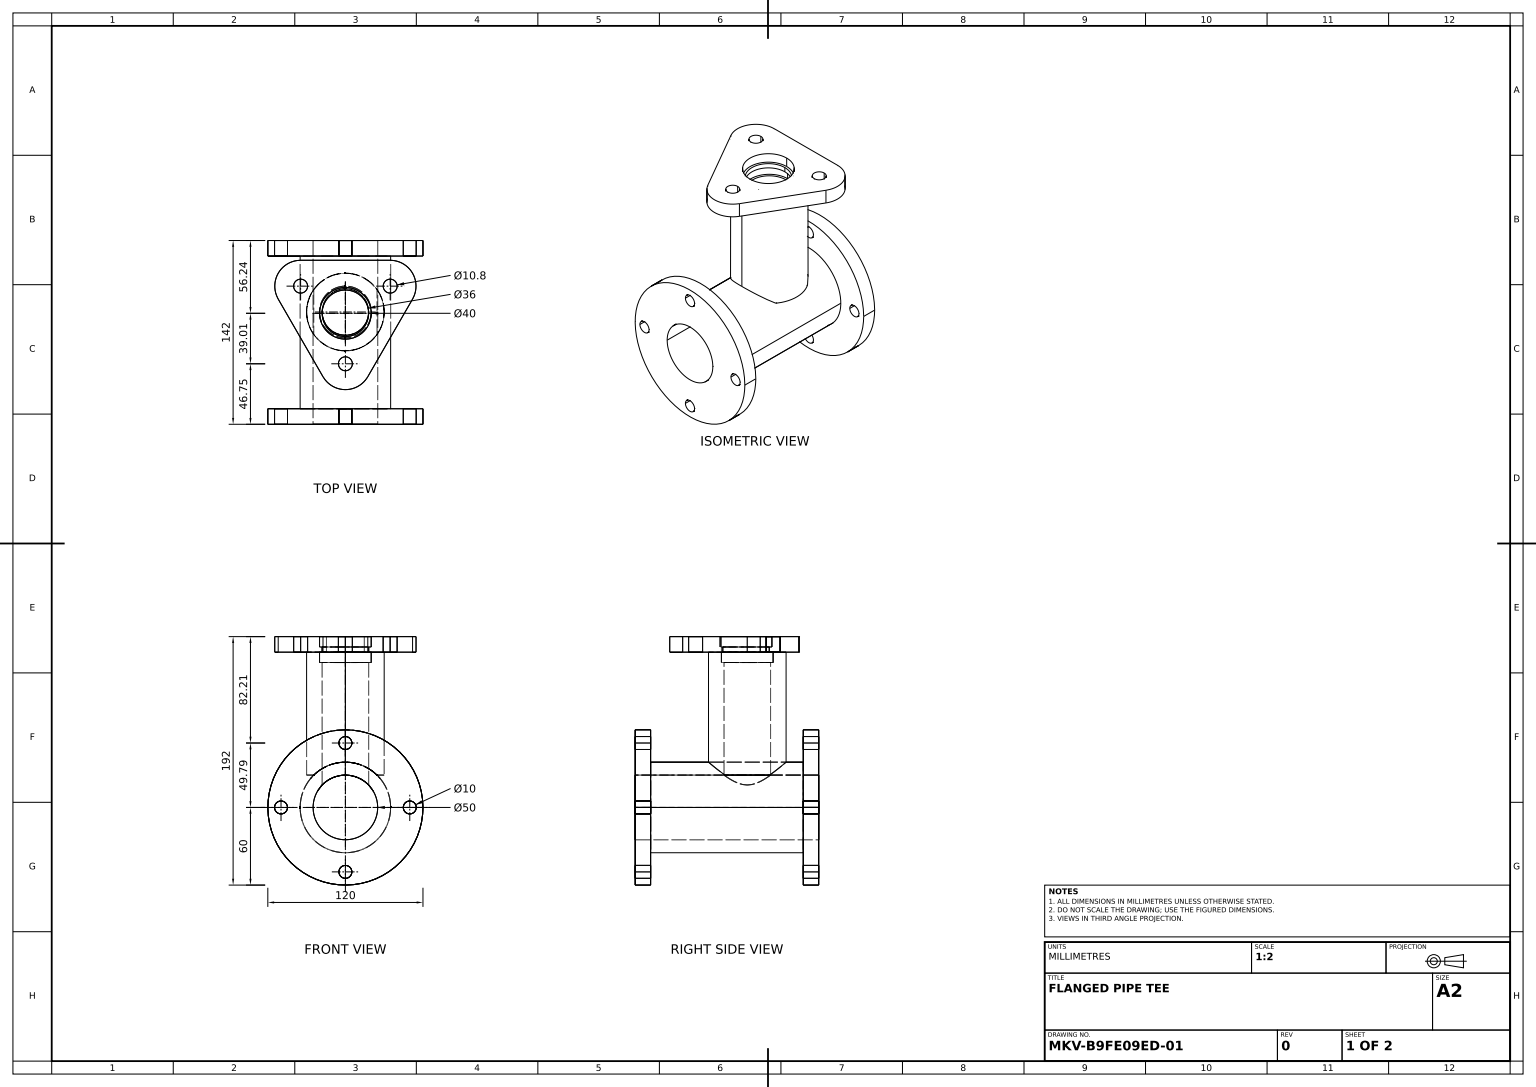
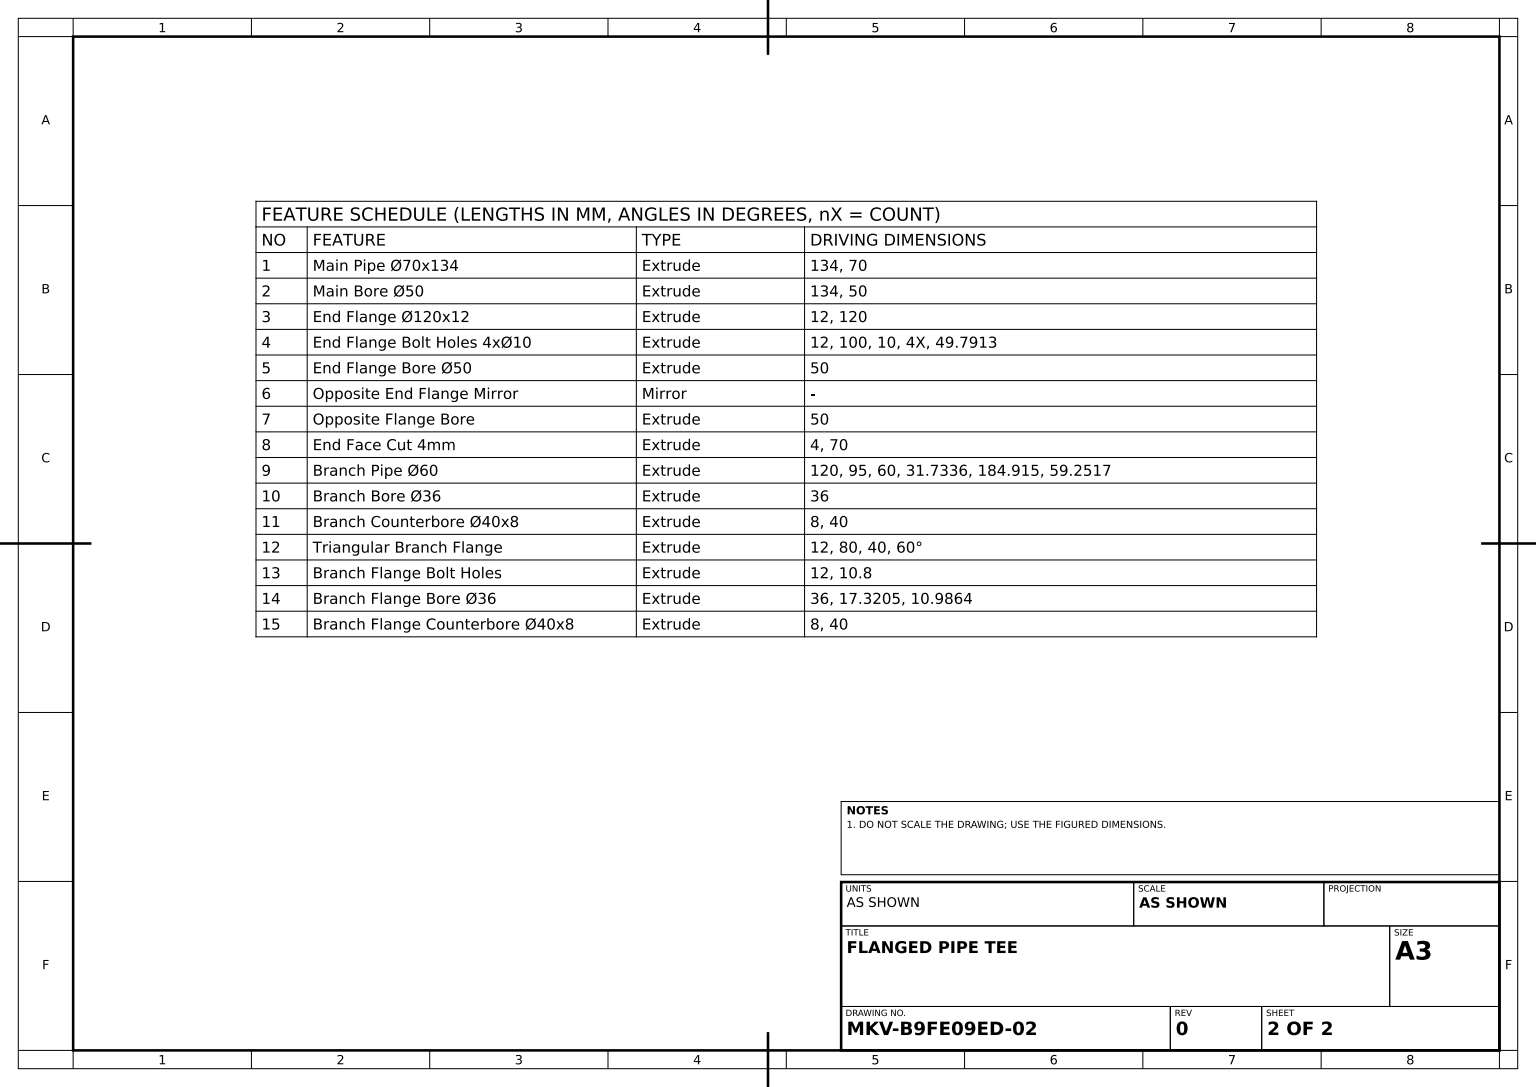
SolidWorks part; units mm, degrees
material "Plain Carbon Steel"
ref_plane "Front Plane" through (0, 0, 0) normal (0, 0, 1) x (1, 0, 0)
ref_plane "Top Plane" through (0, 0, 0) normal (0, 1, 0) x (1, 0, 0)
ref_plane "Right Plane" through (0, 0, 0) normal (1, 0, 0) x (0, 0, -1)
sketch "Main Pipe Sketch" plane through (0, 0, 0) normal (0, 0, 1) x (1, 0, 0)
  line L0 (0, 84.6905) -> (0, -91.4754) construction
  line L1 (-128.9137, 0) -> (134.9717, 0) construction
  circle A0 centre (0, 0) radius 35
  dimension "D1" = 70
extrude "Main Pipe Ø70x134" add sketch "Main Pipe Sketch" along normal blind 134
sketch "Main Bore Sketch" plane through (0, 0, 134) normal (0, 0, 1) x (1, 0, 0)
  circle A0 centre (0, 0) radius 25
  dimension "D1" = 50
extrude "Main Bore Ø50" cut sketch "Main Bore Sketch" against normal blind 134
sketch "End Flange Sketch" plane through (0, 0, 134) normal (0, 0, 1) x (1, 0, 0)
  circle A0 centre (0, 0) radius 60
  dimension "D1" = 120
extrude "End Flange Ø120x12" add sketch "End Flange Sketch" along normal blind 12
sketch "End Flange Bolt Holes Sketch" plane through (0, 0, 146) normal (0, 0, 1) x (1, 0, 0)
  line L0 (0, 80.5312) -> (0, -84.6861) construction
  circle A0 centre (0, 0) radius 50 construction
  circle A1 centre (0, 49.7913) radius 5
  circle A2 centre (49.7913, 0) radius 5
  circle A3 centre (0, -49.7913) radius 5
  circle A4 centre (-49.7913, 0) radius 5
  circle A5 centre (0, 0) radius 60 construction
  point P16 (0, 0)
  dimension "D1" = 100
  dimension "D2" = 10
  dimension "D4" = 49.7913
  dimension "D3" = 4
extrude "End Flange Bolt Holes 4xØ10" cut sketch "End Flange Bolt Holes Sketch" against normal blind 12
sketch "End Flange Bore Sketch" plane through (0, 0, 146) normal (0, 0, 1) x (1, 0, 0)
  circle A0 centre (0, 0) radius 25
  dimension "D1" = 50
extrude "End Flange Bore Ø50" cut sketch "End Flange Bore Sketch" against normal through all
ref_plane "Plane1" through (0, 0, 75) normal (0, 0, 1) x (1, 0, 0)
mirror "Opposite End Flange Mirror" about plane through (0, 0, 75) normal (0, 0, 1) of "End Flange Bolt Holes 4xØ10", "End Flange Ø120x12"
sketch "Opposite Flange Bore Sketch" plane through (0, 0, 4) normal (0, 0, -1) x (-1, 0, 0)
  circle A0 centre (0, 0) radius 25
  dimension "D1" = 50
extrude "Opposite Flange Bore" cut sketch "Opposite Flange Bore Sketch" against normal through all
sketch "End Face Cut Sketch" plane through (0, 0, 0) normal (0, 0, -1) x (-1, 0, 0)
  circle A0 centre (0, 0) radius 35
  dimension "D1" = 70
extrude "End Face Cut 4mm" cut sketch "End Face Cut Sketch" against normal blind 4
ref_plane "Plane3" through (0, 120, 0) normal (0, 1, 0) x (1, 0, 0)
sketch "Branch Pipe Sketch" plane through (0, 120, 0) normal (0, 1, 0) x (1, 0, 0)
  line L0 (0, 31.7336) -> (0, -184.915) construction
  circle A0 centre (0, -59.2517) radius 30
  dimension "D3" = 60
  dimension "D1" = 31.7336
  dimension "D2" = 184.915
  dimension "D4" = 59.2517
extrude "Branch Pipe Ø60" add sketch "Branch Pipe Sketch" against normal blind 95
sketch "Branch Bore Sketch" plane through (0, 120, 0) normal (0, 1, 0) x (1, 0, 0)
  circle A0 centre (0, -59.2517) radius 18
  dimension "D1" = 36
extrude "Branch Bore Ø36" cut sketch "Branch Bore Sketch" against normal up to next contours A0
sketch "Branch Counterbore Sketch" plane through (0, 120, 0) normal (0, 1, 0) x (1, 0, 0)
  circle A0 centre (0, -59.2517) radius 20
  dimension "D1" = 40
extrude "Branch Counterbore Ø40x8" cut sketch "Branch Counterbore Sketch" against normal blind 8
sketch "Branch Flange Sketch" plane through (0, 120, 0) normal (0, 1, 0) x (1, 0, 0)
  line L0 (0, 37.6191) -> (0, -163.6723) construction
  line L1 (0, -59.2517) -> (-77.5982, -14.4504) construction
  line L2 (-51.9615, -49.2517) -> (-17.3205, -109.2517)
  line L3 (-34.641, -19.2517) -> (34.641, -19.2517)
  line L4 (51.9615, -49.2517) -> (17.3205, -109.2517)
  circle A0 centre (0, -59.2517) radius 40 construction
  arc A1 (-17.3205, -109.2517) -> (17.3205, -109.2517) centre (0, -99.2517) ccw
  arc A2 (-34.641, -19.2517) -> (-51.9615, -49.2517) centre (-34.641, -39.2517) ccw
  arc A3 (34.641, -19.2517) -> (51.9615, -49.2517) centre (34.641, -39.2517) cw
  dimension "D1" = 80
  dimension "D2" = 40
  dimension "D4" = 40
  dimension "D3" = 60
extrude "Triangular Branch Flange" add sketch "Branch Flange Sketch" along normal blind 12
sketch "Branch Flange Holes Sketch" plane through (0, 132, 0) normal (0, 1, 0) x (1, 0, 0)
  line L0 (0, 30.7069) -> (0, -165.9571) construction
  circle A0 centre (-34.641, -39.2517) radius 5.4
  circle A1 centre (34.641, -39.2517) radius 5.4
  circle A2 centre (0, -99.2517) radius 5.4
  dimension "D1" = 10.8
  dimension "D2" = 10.8
extrude "Branch Flange Bolt Holes" cut sketch "Branch Flange Holes Sketch" against normal blind 12
sketch "Branch Flange Bore Sketch" plane through (0, 132, 0) normal (0, 1, 0) x (1, 0, 0)
  circle A0 centre (0, -60.2381) radius 18
  dimension "D1" = 36
  dimension "D2" = 17.3205
  dimension "D3" = 10.9864
extrude "Branch Flange Bore Ø36" cut sketch "Branch Flange Bore Sketch" against normal up to next
sketch "Branch Flange Counterbore Sketch" plane through (0, 132, 0) normal (0, 1, 0) x (1, 0, 0)
  circle A0 centre (0, -60.2381) radius 20
  dimension "D1" = 40
extrude "Branch Flange Counterbore Ø40x8" cut sketch "Branch Flange Counterbore Sketch" against normal blind 8
